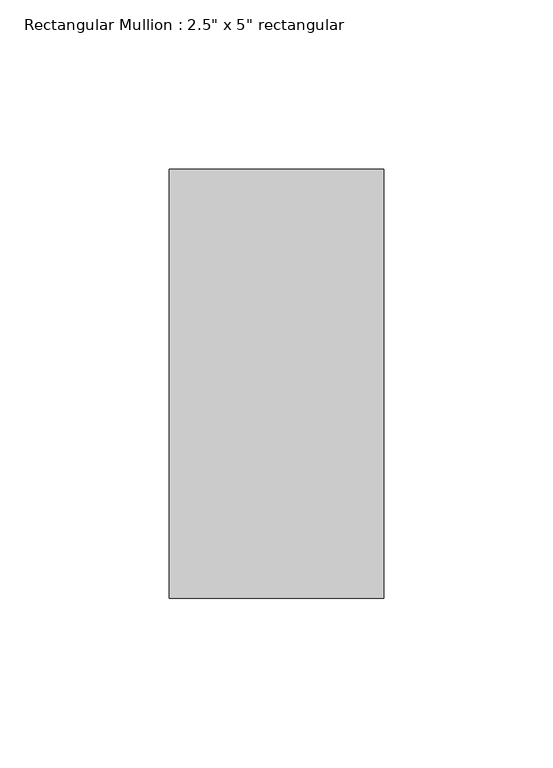
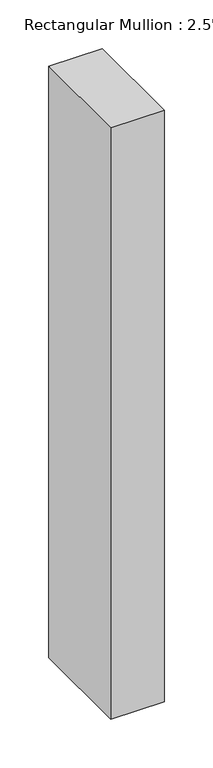
"""IFC4 building model written with IfcOpenShell, lengths in millimetres: member geometry."""

from ifc_helpers import new_model, si_unit, frame, origin, place, context, project, spatial, polyline, outline, extrude, source, transform, mapped, element, save


def member_510dacbd(model_context):
    return source(origin(), model_context, "Body", "SweptSolid", [
        extrude(outline(polyline([(0.0, 63.5), (0.0, -63.5), (-63.5, -63.5), (-63.5, 63.5), (0.0, 63.5)])), frame((0.0, 0.0, -741.4158453), z_axis=(0.0, 0.0, 1.0), x_axis=(1.0, 0.0, 0.0)), (0.0, 0.0, 1.0), 741.4158453),
    ])


if __name__ == "__main__":
    model = new_model("IFC4")
    model_context = context("Model", 3, world=origin())
    ifc_project = project(units=[si_unit("LENGTHUNIT", "METRE", prefix="MILLI")], contexts=[model_context])
    site = spatial("IfcSite", under=ifc_project)
    building = spatial("IfcBuilding", under=site)
    placement = place(None, origin())
    member_shape = member_510dacbd(model_context)
    element("IfcMember", 1, ObjectType="Rectangular Mullion : 2.5\" x 5\" rectangular", at=placement, inside=building, context=model_context, shape_type="MappedRepresentation", body=[
        mapped(member_shape, transform((0.0, 0.0, 0.0), x_axis=(1.0, 0.0, 0.0), y_axis=(0.0, 1.0, 0.0), z_axis=(0.0, 0.0, 1.0))),
    ])
    save(model, "model.ifc")

# Revit data of these elements
# Type "Rectangular Mullion : 2.5\" x 5\" rectangular"
#   built-in parameter 1007304 = 0.416667 (stored number, unit not read)
#   built-in parameter 1007301 = 0.104167 (stored number, unit not read)
#   built-in parameter 1007300 = 0.104167 (stored number, unit not read)
# Element 1 (IfcMember, "Rectangular Mullion : 2.5\" x 5\" rectangular")
#   Materials on its faces: "Aluminum"
# Materials
#   "Aluminum": class "Metal", colour RGB 247 247 247, transparency 0, Description = "Aluminum 6061", Cost = 0
